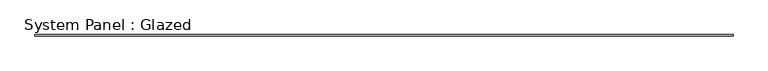
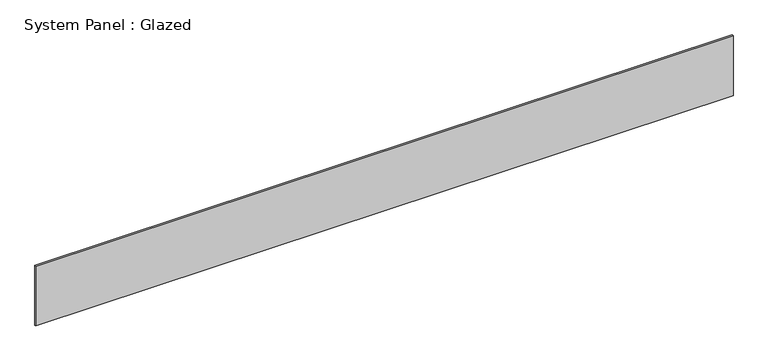
"""IFC4 building model written with IfcOpenShell, lengths in millimetres: plate geometry, System Panel : Glazed."""

from ifc_helpers import new_model, si_unit, origin, origin_with_axes, place, context, project, spatial, polyline, outline, extrude, source, transform, mapped, element, save


def system_panel_glazed_1f2476a4(model_context):
    return source(origin(), model_context, "Body", "SweptSolid", [
        extrude(outline(polyline([(6370.2331637, 19.05), (-6370.2331637, 19.05), (-6370.2331637, 44.45), (6370.2331637, 44.45), (6370.2331637, 19.05)])), origin_with_axes(), (0.0, 0.0, 1.0), 1155.7),
    ])


if __name__ == "__main__":
    model = new_model("IFC4")
    model_context = context("Model", 3, world=origin())
    ifc_project = project(units=[si_unit("LENGTHUNIT", "METRE", prefix="MILLI")], contexts=[model_context])
    site = spatial("IfcSite", under=ifc_project)
    building = spatial("IfcBuilding", under=site)
    placement = place(None, origin())
    system_panel_glazed_shape = system_panel_glazed_1f2476a4(model_context)
    element("IfcPlate", 1, ObjectType="System Panel : Glazed", at=placement, inside=building, context=model_context, shape_type="MappedRepresentation", body=[
        mapped(system_panel_glazed_shape, transform((0.0, 0.0, 0.0), x_axis=(1.0, 0.0, 0.0), y_axis=(0.0, 1.0, 0.0), z_axis=(0.0, 0.0, 1.0))),
    ])
    save(model, "model.ifc")

# Revit data of these elements
# Type "System Panel : Glazed"
#   Construction Type Id = "GSP4R"
#   Analytic Construction = "1/8 in Pilkington single glazing"
#   Visual Light Transmittance = 0.9
#   Solar Heat Gain Coefficient = 0.86
#   Heat Transfer Coefficient (U) = 1.18115 BTU/(h·ft²·°F)
# Element 1 (IfcPlate, "System Panel : Glazed")
#   Materials on its faces: "Glass"
# Materials
#   "Glass": class "Glass", colour RGB 0 128 192, transparency 0.75, Description = "Soda Lime Glass", Cost = 0
